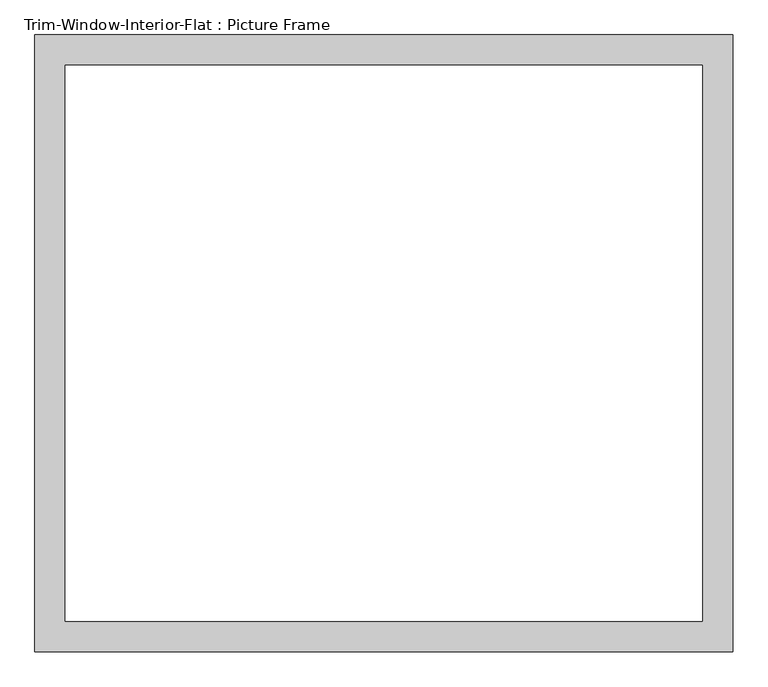
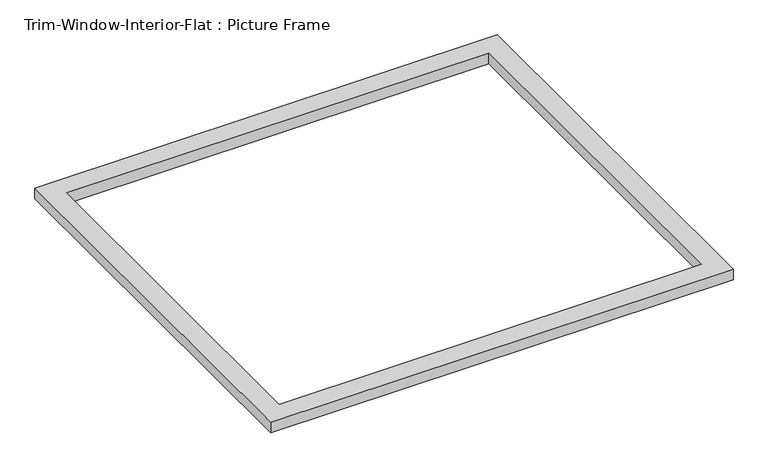
"""IFC4 building model written with IfcOpenShell, lengths in millimetres: proxy geometry, Trim-Window-Interior-Flat : Picture Frame."""

from ifc_helpers import new_model, si_unit, origin, origin_with_axes, place, context, project, spatial, polyline, outline, extrude, source, transform, mapped, element, save


def trim_window_interior_flat_picture_frame_1dce1945(model_context):
    return source(origin(), model_context, "Body", "SweptSolid", [
        extrude(outline(polyline([(654.05, 44.45), (654.05, -1111.25), (-654.05, -1111.25), (-654.05, 44.45), (654.05, 44.45)]), holes=[polyline([(596.9, -12.7), (-596.9, -12.7), (-596.9, -1054.1), (596.9, -1054.1), (596.9, -12.7)])]), origin_with_axes(), (0.0, 0.0, 1.0), 31.75),
    ])


if __name__ == "__main__":
    model = new_model("IFC4")
    model_context = context("Model", 3, world=origin())
    ifc_project = project(units=[si_unit("LENGTHUNIT", "METRE", prefix="MILLI")], contexts=[model_context])
    site = spatial("IfcSite", under=ifc_project)
    building = spatial("IfcBuilding", under=site)
    placement = place(None, origin())
    trim_window_interior_flat_picture_frame_shape = trim_window_interior_flat_picture_frame_1dce1945(model_context)
    element("IfcBuildingElementProxy", 1, Name="Trim-Window-Interior-Flat : Picture Frame", ObjectType="Trim-Window-Interior-Flat : Picture Frame", at=placement, inside=building, context=model_context, shape_type="MappedRepresentation", body=[
        mapped(trim_window_interior_flat_picture_frame_shape, transform((0.0, 0.0, 0.0), x_axis=(1.0, 0.0, 0.0), y_axis=(0.0, 1.0, 0.0), z_axis=(0.0, 0.0, 1.0))),
    ])
    save(model, "model.ifc")

# Revit data of these elements
# Type "Trim-Window-Interior-Flat : Picture Frame"
#   Trim Thickness_Picture Frame = 0' - 1 1/4"
#   Trim Width = 0' - 2 1/4"
#   Trim Thickness_with Sill = 0' - 0 3/4"
#   Sill Thickness = 0' - 1 1/4"
#   Opening Width [instance default] = 2' - 0"
#   Opening Height [instance default] = 3' - 0"
#   Default Elevation = 4' - 0"
#   Sill = no
#   Picture Frame = yes
#   Trim Material [instance default] = none
# Element 1 (IfcBuildingElementProxy, "Trim-Window-Interior-Flat : Picture Frame")
#   Opening Width = 4' - 0"
#   Opening Height = 3' - 6"
#   Trim Material = Wood - Stained
#   Materials on its faces: "Wood - Stained"
# Materials
#   "Wood - Stained": class "Wood", colour RGB 224 178 126, transparency 0, Cost = 0
